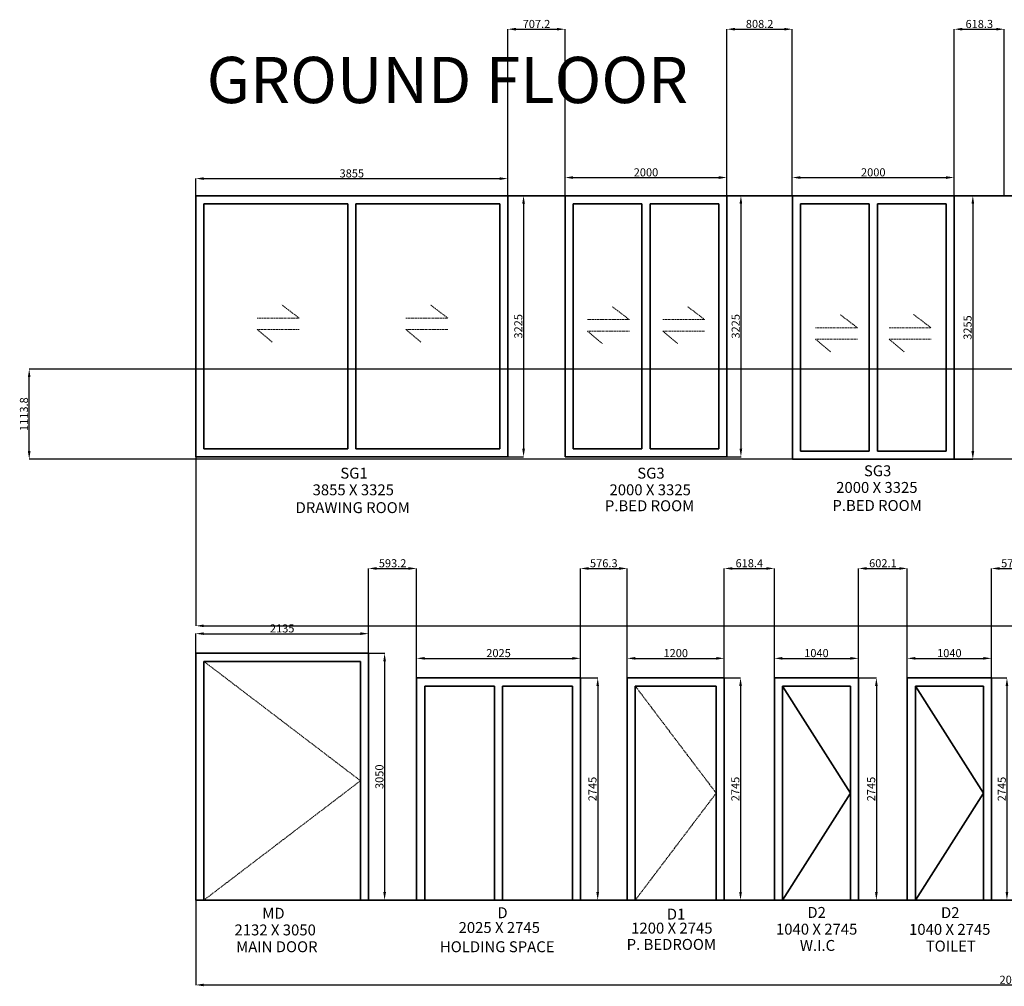
# Model space of a CAD drawing. Units: millimetres. Extents: x -850 to 42148, y -7352 to 4589.
# Tile 1 of 4: x -850 to 11314, y -7352 to 4589. Entities that reach past the tile are written whole.
import ezdxf

# ---------------------------------------------------------------- set-up
doc = ezdxf.new("R2010")
doc.units = ezdxf.units.MM
doc.linetypes.add('DASHED', pattern=[19.05, 12.7, -6.35])
for name, color, linetype, lineweight in [('A-ANNO-DIMS', 2, 'Continuous', 18), ('A-ANNO-TEXT', 7, 'Continuous', 18), ('A-DOOR', 3, 'Continuous', 35), ('A-DOOR-OPNG', 3, 'DASHED', 18), ('A-GLAZ', 4, 'Continuous', 35), ('A-GLAZ-OPNG', 4, 'DASHED', 18)]:
    doc.layers.add(name, color=color, linetype=linetype, lineweight=lineweight)
doc.styles.get("Standard").update_dxf_attribs({"font": 'arial.ttf'})
doc.dimstyles.new('ISO-25', dxfattribs={"dimtxt": 100, "dimasz": 100, "dimexe": 1.25, "dimexo": 0.625, "dimtad": 1, "dimtxsty": 'Standard', "dimcen": 2.5, "dimadec": 0, "dimazin": 0, "dimtfac": 1, "dimtmove": 0, "dimatfit": 3, "dimfxl": 1, "dimarcsym": 0})

# ---------------------------------------------------------------- blocks, each defined once
blk = doc.blocks.new('*D1')
at = {"layer": 'A-ANNO-DIMS', "color": 0, "lineweight": -2, "transparency": 16777216}
for p, q in [((1325, 2415), (1325, 2627)), ((1425, 2626), (5080, 2626)), ((5180, 2415), (5180, 2627))]:
    blk.add_line(p, q, dxfattribs=at)
at = {"layer": 'A-ANNO-DIMS', "color": 0, "lineweight": 30, "transparency": 16777216}
for points in [[(1425, 2642), (1425, 2609), (1325, 2626)], [(5080, 2642), (5080, 2609), (5180, 2626)]]:
    blk.add_solid(points, dxfattribs=at)
at = {"layer": 'Defpoints', "color": 0, "lineweight": 30, "transparency": 16777216}
for p in [(5180, 2626), (1325, 2414), (5180, 2414)]:
    blk.add_point(p, dxfattribs=at)
at = {"layer": 'A-ANNO-DIMS', "color": 0, "transparency": 16777216, "insert": (3253, 2677), "char_height": 100, "attachment_point": 5}
blk.add_mtext('3855', dxfattribs=at)
blk = doc.blocks.new('*D2')
at = {"layer": 'A-ANNO-DIMS', "color": 0, "lineweight": -2, "transparency": 16777216}
for p, q in [((5181, 2414), (5376, 2414)), ((5375, 2314), (5375, -711)), ((5181, -811), (5376, -811))]:
    blk.add_line(p, q, dxfattribs=at)
at = {"layer": 'A-ANNO-DIMS', "color": 0, "lineweight": 30, "transparency": 16777216}
for points in [[(5358, 2314), (5392, 2314), (5375, 2414)], [(5358, -711), (5392, -711), (5375, -811)]]:
    blk.add_solid(points, dxfattribs=at)
at = {"layer": 'Defpoints', "color": 0, "lineweight": 30, "transparency": 16777216}
for p in [(5180, 2414), (5180, -811), (5375, -811)]:
    blk.add_point(p, dxfattribs=at)
at = {"layer": 'A-ANNO-DIMS', "color": 0, "transparency": 16777216, "insert": (5323, 801), "char_height": 100, "attachment_point": 5, "rotation": 90}
blk.add_mtext('3225', dxfattribs=at)
blk = doc.blocks.new('*D3')
at = {"layer": 'A-ANNO-DIMS', "color": 0, "lineweight": -2, "transparency": 16777216}
for p, q in [((5887, 2415), (5887, 2640)), ((5987, 2639), (7787, 2639)), ((7887, 2415), (7887, 2640))]:
    blk.add_line(p, q, dxfattribs=at)
at = {"layer": 'A-ANNO-DIMS', "color": 0, "lineweight": 30, "transparency": 16777216}
for points in [[(5987, 2655), (5987, 2622), (5887, 2639)], [(7787, 2655), (7787, 2622), (7887, 2639)]]:
    blk.add_solid(points, dxfattribs=at)
at = {"layer": 'Defpoints', "color": 0, "lineweight": 30, "transparency": 16777216}
for p in [(7887, 2639), (5887, 2414), (7887, 2414)]:
    blk.add_point(p, dxfattribs=at)
at = {"layer": 'A-ANNO-DIMS', "color": 0, "transparency": 16777216, "insert": (6887, 2690), "char_height": 100, "attachment_point": 5}
blk.add_mtext('2000', dxfattribs=at)
blk = doc.blocks.new('*D4')
at = {"layer": 'A-ANNO-DIMS', "color": 0, "lineweight": -2, "transparency": 16777216}
for p, q in [((7888, 2414), (8061, 2414)), ((8060, 2314), (8060, -711)), ((7888, -811), (8061, -811))]:
    blk.add_line(p, q, dxfattribs=at)
at = {"layer": 'A-ANNO-DIMS', "color": 0, "lineweight": 30, "transparency": 16777216}
for points in [[(8043, 2314), (8076, 2314), (8060, 2414)], [(8043, -711), (8076, -711), (8060, -811)]]:
    blk.add_solid(points, dxfattribs=at)
at = {"layer": 'Defpoints', "color": 0, "lineweight": 30, "transparency": 16777216}
for p in [(7887, 2414), (7887, -811), (8060, -811)]:
    blk.add_point(p, dxfattribs=at)
at = {"layer": 'A-ANNO-DIMS', "color": 0, "transparency": 16777216, "insert": (8008, 801), "char_height": 100, "attachment_point": 5, "rotation": 90}
blk.add_mtext('3225', dxfattribs=at)
blk = doc.blocks.new('*D5')
at = {"layer": 'A-ANNO-DIMS', "color": 0, "lineweight": -2, "transparency": 16777216}
for p, q in [((8695, 2415), (8695, 2640)), ((8795, 2639), (10595, 2639)), ((10695, 2415), (10695, 2640))]:
    blk.add_line(p, q, dxfattribs=at)
at = {"layer": 'A-ANNO-DIMS', "color": 0, "lineweight": 30, "transparency": 16777216}
for points in [[(8795, 2655), (8795, 2622), (8695, 2639)], [(10595, 2655), (10595, 2622), (10695, 2639)]]:
    blk.add_solid(points, dxfattribs=at)
at = {"layer": 'Defpoints', "color": 0, "lineweight": 30, "transparency": 16777216}
for p in [(10695, 2639), (8695, 2414), (10695, 2414)]:
    blk.add_point(p, dxfattribs=at)
at = {"layer": 'A-ANNO-DIMS', "color": 0, "transparency": 16777216, "insert": (9695, 2690), "char_height": 100, "attachment_point": 5}
blk.add_mtext('2000', dxfattribs=at)
blk = doc.blocks.new('*D6')
at = {"layer": 'A-ANNO-DIMS', "color": 0, "lineweight": -2, "transparency": 16777216}
for p, q in [((10696, 2414), (10926, 2414)), ((10925, 2314), (10925, -741)), ((10696, -841), (10926, -841))]:
    blk.add_line(p, q, dxfattribs=at)
at = {"layer": 'A-ANNO-DIMS', "color": 0, "lineweight": 30, "transparency": 16777216}
for points in [[(10908, 2314), (10942, 2314), (10925, 2414)], [(10908, -741), (10942, -741), (10925, -841)]]:
    blk.add_solid(points, dxfattribs=at)
at = {"layer": 'Defpoints', "color": 0, "lineweight": 30, "transparency": 16777216}
for p in [(10695, 2414), (10695, -841), (10925, -841)]:
    blk.add_point(p, dxfattribs=at)
at = {"layer": 'A-ANNO-DIMS', "color": 0, "transparency": 16777216, "insert": (10873, 786), "char_height": 100, "attachment_point": 5, "rotation": 90}
blk.add_mtext('3255', dxfattribs=at)
blk = doc.blocks.new('*D29')
at = {"layer": 'A-ANNO-DIMS', "color": 0, "lineweight": -2, "transparency": 16777216}
for p, q in [((1325, -3237), (1325, -2994)), ((1425, -2996), (3360, -2996)), ((3460, -3237), (3460, -2994))]:
    blk.add_line(p, q, dxfattribs=at)
at = {"layer": 'A-ANNO-DIMS', "color": 0, "lineweight": 30, "transparency": 16777216}
for points in [[(1425, -2979), (1425, -3012), (1325, -2996)], [(3360, -2979), (3360, -3012), (3460, -2996)]]:
    blk.add_solid(points, dxfattribs=at)
at = {"layer": 'Defpoints', "color": 0, "lineweight": 30, "transparency": 16777216}
for p in [(3460, -2996), (1325, -3238), (3460, -3238)]:
    blk.add_point(p, dxfattribs=at)
at = {"layer": 'A-ANNO-DIMS', "color": 0, "transparency": 16777216, "insert": (2393, -2944), "char_height": 100, "attachment_point": 5}
blk.add_mtext('2135', dxfattribs=at)
blk = doc.blocks.new('*D30')
at = {"layer": 'A-ANNO-DIMS', "color": 0, "lineweight": -2, "transparency": 16777216}
for p, q in [((3461, -3238), (3660, -3238)), ((3658, -3338), (3658, -6188)), ((3461, -6288), (3660, -6288))]:
    blk.add_line(p, q, dxfattribs=at)
at = {"layer": 'A-ANNO-DIMS', "color": 0, "lineweight": 30, "transparency": 16777216}
for points in [[(3642, -3338), (3675, -3338), (3658, -3238)], [(3642, -6188), (3675, -6188), (3658, -6288)]]:
    blk.add_solid(points, dxfattribs=at)
at = {"layer": 'Defpoints', "color": 0, "lineweight": 30, "transparency": 16777216}
for p in [(3460, -3238), (3460, -6288), (3658, -6288)]:
    blk.add_point(p, dxfattribs=at)
at = {"layer": 'A-ANNO-DIMS', "color": 0, "transparency": 16777216, "insert": (3607, -4763), "char_height": 100, "attachment_point": 5, "rotation": 90}
blk.add_mtext('3050', dxfattribs=at)
blk = doc.blocks.new('*D31')
at = {"layer": 'A-ANNO-DIMS', "color": 0, "lineweight": -2, "transparency": 16777216}
for p, q in [((4053, -3542), (4053, -3299)), ((4153, -3301), (5978, -3301)), ((6078, -3542), (6078, -3299))]:
    blk.add_line(p, q, dxfattribs=at)
at = {"layer": 'A-ANNO-DIMS', "color": 0, "lineweight": 30, "transparency": 16777216}
for points in [[(4153, -3284), (4153, -3317), (4053, -3301)], [(5978, -3284), (5978, -3317), (6078, -3301)]]:
    blk.add_solid(points, dxfattribs=at)
at = {"layer": 'Defpoints', "color": 0, "lineweight": 30, "transparency": 16777216}
for p in [(6078, -3301), (4053, -3543), (6078, -3543)]:
    blk.add_point(p, dxfattribs=at)
at = {"layer": 'A-ANNO-DIMS', "color": 0, "transparency": 16777216, "insert": (5066, -3249), "char_height": 100, "attachment_point": 5}
blk.add_mtext('2025', dxfattribs=at)
blk = doc.blocks.new('*D32')
at = {"layer": 'A-ANNO-DIMS', "color": 0, "lineweight": -2, "transparency": 16777216}
for p, q in [((6079, -3543), (6292, -3543)), ((6291, -3643), (6291, -6188)), ((6079, -6288), (6292, -6288))]:
    blk.add_line(p, q, dxfattribs=at)
at = {"layer": 'A-ANNO-DIMS', "color": 0, "lineweight": 30, "transparency": 16777216}
for points in [[(6274, -3643), (6307, -3643), (6291, -3543)], [(6274, -6188), (6307, -6188), (6291, -6288)]]:
    blk.add_solid(points, dxfattribs=at)
at = {"layer": 'Defpoints', "color": 0, "lineweight": 30, "transparency": 16777216}
for p in [(6078, -3543), (6078, -6288), (6291, -6288)]:
    blk.add_point(p, dxfattribs=at)
at = {"layer": 'A-ANNO-DIMS', "color": 0, "transparency": 16777216, "insert": (6239, -4915), "char_height": 100, "attachment_point": 5, "rotation": 90}
blk.add_mtext('2745', dxfattribs=at)
blk = doc.blocks.new('*D33')
at = {"layer": 'A-ANNO-DIMS', "color": 0, "lineweight": -2, "transparency": 16777216}
for p, q in [((6655, -3542), (6655, -3299)), ((6755, -3301), (7755, -3301)), ((7855, -3542), (7855, -3299))]:
    blk.add_line(p, q, dxfattribs=at)
at = {"layer": 'A-ANNO-DIMS', "color": 0, "lineweight": 30, "transparency": 16777216}
for points in [[(6755, -3284), (6755, -3317), (6655, -3301)], [(7755, -3284), (7755, -3317), (7855, -3301)]]:
    blk.add_solid(points, dxfattribs=at)
at = {"layer": 'Defpoints', "color": 0, "lineweight": 30, "transparency": 16777216}
for p in [(7855, -3301), (6655, -3543), (7855, -3543)]:
    blk.add_point(p, dxfattribs=at)
at = {"layer": 'A-ANNO-DIMS', "color": 0, "transparency": 16777216, "insert": (7255, -3249), "char_height": 100, "attachment_point": 5}
blk.add_mtext('1200', dxfattribs=at)
blk = doc.blocks.new('*D34')
at = {"layer": 'A-ANNO-DIMS', "color": 0, "lineweight": -2, "transparency": 16777216}
for p, q in [((7855, -3543), (8056, -3543)), ((8055, -3643), (8055, -6188)), ((7855, -6288), (8056, -6288))]:
    blk.add_line(p, q, dxfattribs=at)
at = {"layer": 'A-ANNO-DIMS', "color": 0, "lineweight": 30, "transparency": 16777216}
for points in [[(8039, -3643), (8072, -3643), (8055, -3543)], [(8039, -6188), (8072, -6188), (8055, -6288)]]:
    blk.add_solid(points, dxfattribs=at)
at = {"layer": 'Defpoints', "color": 0, "lineweight": 30, "transparency": 16777216}
for p in [(7855, -3543), (7855, -6288), (8055, -6288)]:
    blk.add_point(p, dxfattribs=at)
at = {"layer": 'A-ANNO-DIMS', "color": 0, "transparency": 16777216, "insert": (8004, -4915), "char_height": 100, "attachment_point": 5, "rotation": 90}
blk.add_mtext('2745', dxfattribs=at)
blk = doc.blocks.new('*D35')
at = {"layer": 'A-ANNO-DIMS', "color": 0, "lineweight": -2, "transparency": 16777216}
for p, q in [((8473, -3542), (8473, -3299)), ((8573, -3301), (9413, -3301)), ((9513, -3542), (9513, -3299))]:
    blk.add_line(p, q, dxfattribs=at)
at = {"layer": 'A-ANNO-DIMS', "color": 0, "lineweight": 30, "transparency": 16777216}
for points in [[(8573, -3284), (8573, -3317), (8473, -3301)], [(9413, -3284), (9413, -3317), (9513, -3301)]]:
    blk.add_solid(points, dxfattribs=at)
at = {"layer": 'Defpoints', "color": 0, "lineweight": 30, "transparency": 16777216}
for p in [(9513, -3301), (8473, -3543), (9513, -3543)]:
    blk.add_point(p, dxfattribs=at)
at = {"layer": 'A-ANNO-DIMS', "color": 0, "transparency": 16777216, "insert": (8993, -3249), "char_height": 100, "attachment_point": 5}
blk.add_mtext('1040', dxfattribs=at)
blk = doc.blocks.new('*D36')
at = {"layer": 'A-ANNO-DIMS', "color": 0, "lineweight": -2, "transparency": 16777216}
for p, q in [((9514, -3543), (9735, -3543)), ((9733, -3643), (9733, -6188)), ((9514, -6288), (9735, -6288))]:
    blk.add_line(p, q, dxfattribs=at)
at = {"layer": 'A-ANNO-DIMS', "color": 0, "lineweight": 30, "transparency": 16777216}
for points in [[(9717, -3643), (9750, -3643), (9733, -3543)], [(9717, -6188), (9750, -6188), (9733, -6288)]]:
    blk.add_solid(points, dxfattribs=at)
at = {"layer": 'Defpoints', "color": 0, "lineweight": 30, "transparency": 16777216}
for p in [(9513, -3543), (9513, -6288), (9733, -6288)]:
    blk.add_point(p, dxfattribs=at)
at = {"layer": 'A-ANNO-DIMS', "color": 0, "transparency": 16777216, "insert": (9682, -4915), "char_height": 100, "attachment_point": 5, "rotation": 90}
blk.add_mtext('2745', dxfattribs=at)
blk = doc.blocks.new('*D37')
at = {"layer": 'A-ANNO-DIMS', "color": 0, "lineweight": -2, "transparency": 16777216}
for p, q in [((10115, -3542), (10115, -3299)), ((10215, -3301), (11055, -3301)), ((11155, -3542), (11155, -3299))]:
    blk.add_line(p, q, dxfattribs=at)
at = {"layer": 'A-ANNO-DIMS', "color": 0, "lineweight": 30, "transparency": 16777216}
for points in [[(10215, -3284), (10215, -3317), (10115, -3301)], [(11055, -3284), (11055, -3317), (11155, -3301)]]:
    blk.add_solid(points, dxfattribs=at)
at = {"layer": 'Defpoints', "color": 0, "lineweight": 30, "transparency": 16777216}
for p in [(11155, -3301), (10115, -3543), (11155, -3543)]:
    blk.add_point(p, dxfattribs=at)
at = {"layer": 'A-ANNO-DIMS', "color": 0, "transparency": 16777216, "insert": (10635, -3249), "char_height": 100, "attachment_point": 5}
blk.add_mtext('1040', dxfattribs=at)
blk = doc.blocks.new('*D38')
at = {"layer": 'A-ANNO-DIMS', "color": 0, "lineweight": -2, "transparency": 16777216}
for p, q in [((11156, -3543), (11347, -3543)), ((11346, -3643), (11346, -6188)), ((11156, -6288), (11347, -6288))]:
    blk.add_line(p, q, dxfattribs=at)
at = {"layer": 'A-ANNO-DIMS', "color": 0, "lineweight": 30, "transparency": 16777216}
for points in [[(11330, -3643), (11363, -3643), (11346, -3543)], [(11330, -6188), (11363, -6188), (11346, -6288)]]:
    blk.add_solid(points, dxfattribs=at)
at = {"layer": 'Defpoints', "color": 0, "lineweight": 30, "transparency": 16777216}
for p in [(11155, -3543), (11155, -6288), (11346, -6288)]:
    blk.add_point(p, dxfattribs=at)
at = {"layer": 'A-ANNO-DIMS', "color": 0, "transparency": 16777216, "insert": (11295, -4915), "char_height": 100, "attachment_point": 5, "rotation": 90}
blk.add_mtext('2745', dxfattribs=at)
blk = doc.blocks.new('SYM-SLIDE-ARROW')
for p, q in [((2602, 903), (2388, 1066)), ((2084, 903), (2602, 903)), ((2085, 760), (2604, 760)), ((2085, 760), (2269, 607))]:
    blk.add_line(p, q)
blk = doc.blocks.new('DOOR-D2-1040')
for p, q in [((8473, -6288), (8473, -3543)), ((8473, -3543), (9513, -3543)), ((8573, -6288), (8573, -3643)), ((8573, -3643), (9413, -3643)), ((8573, -3643), (9413, -4965)), ((9413, -3643), (9413, -6288)), ((9513, -3543), (9513, -6288)), ((9413, -4965), (8573, -6288))]:
    blk.add_line(p, q)
blk = doc.blocks.new('*D60')
at = {"layer": 'A-ANNO-DIMS', "color": 0, "lineweight": -2, "transparency": 16777216}
for p, q in [((41489, -432), (41489, -2900)), ((1325, -812), (1325, -2900)), ((1425, -2899), (41389, -2899))]:
    blk.add_line(p, q, dxfattribs=at)
at = {"layer": 'A-ANNO-DIMS', "color": 0, "lineweight": 30, "transparency": 16777216}
for points in [[(1425, -2882), (1425, -2915), (1325, -2899)], [(41389, -2882), (41389, -2915), (41489, -2899)]]:
    blk.add_solid(points, dxfattribs=at)
at = {"layer": 'Defpoints', "color": 0, "lineweight": 30, "transparency": 16777216}
for p in [(41489, -431), (1325, -811), (41489, -2899)]:
    blk.add_point(p, dxfattribs=at)
at = {"layer": 'A-ANNO-DIMS', "color": 0, "transparency": 16777216, "insert": (21407, -2847), "char_height": 100, "attachment_point": 5}
blk.add_mtext('40164', dxfattribs=at)
blk = doc.blocks.new('*D61')
at = {"layer": 'A-ANNO-DIMS', "color": 0, "lineweight": -2, "transparency": 16777216}
for p, q in [((5180, 2415), (5180, 4473)), ((5280, 4471), (5787, 4471)), ((5887, 2415), (5887, 4473))]:
    blk.add_line(p, q, dxfattribs=at)
at = {"layer": 'A-ANNO-DIMS', "color": 0, "lineweight": 30, "transparency": 16777216}
for points in [[(5280, 4488), (5280, 4455), (5180, 4471)], [(5787, 4488), (5787, 4455), (5887, 4471)]]:
    blk.add_solid(points, dxfattribs=at)
at = {"layer": 'Defpoints', "color": 0, "lineweight": 30, "transparency": 16777216}
for p in [(5887, 4471), (5180, 2414), (5887, 2414)]:
    blk.add_point(p, dxfattribs=at)
at = {"layer": 'A-ANNO-DIMS', "color": 0, "transparency": 16777216, "insert": (5534, 4523), "char_height": 100, "attachment_point": 5}
blk.add_mtext('707.2', dxfattribs=at)
blk = doc.blocks.new('*D62')
at = {"layer": 'A-ANNO-DIMS', "color": 0, "lineweight": -2, "transparency": 16777216}
for p, q in [((7887, 2415), (7887, 4473)), ((7987, 4471), (8595, 4471)), ((8695, 2415), (8695, 4473))]:
    blk.add_line(p, q, dxfattribs=at)
at = {"layer": 'A-ANNO-DIMS', "color": 0, "lineweight": 30, "transparency": 16777216}
for points in [[(7987, 4488), (7987, 4455), (7887, 4471)], [(8595, 4488), (8595, 4455), (8695, 4471)]]:
    blk.add_solid(points, dxfattribs=at)
at = {"layer": 'Defpoints', "color": 0, "lineweight": 30, "transparency": 16777216}
for p in [(8695, 4471), (7887, 2414), (8695, 2414)]:
    blk.add_point(p, dxfattribs=at)
at = {"layer": 'A-ANNO-DIMS', "color": 0, "transparency": 16777216, "insert": (8291, 4523), "char_height": 100, "attachment_point": 5}
blk.add_mtext('808.2', dxfattribs=at)
blk = doc.blocks.new('*D63')
at = {"layer": 'A-ANNO-DIMS', "color": 0, "lineweight": -2, "transparency": 16777216}
for p, q in [((10695, 2415), (10695, 4473)), ((10795, 4471), (11214, 4471)), ((11314, 2415), (11314, 4473))]:
    blk.add_line(p, q, dxfattribs=at)
at = {"layer": 'A-ANNO-DIMS', "color": 0, "lineweight": 30, "transparency": 16777216}
for points in [[(10795, 4488), (10795, 4455), (10695, 4471)], [(11214, 4488), (11214, 4455), (11314, 4471)]]:
    blk.add_solid(points, dxfattribs=at)
at = {"layer": 'Defpoints', "color": 0, "lineweight": 30, "transparency": 16777216}
for p in [(11314, 4471), (10695, 2414), (11314, 2414)]:
    blk.add_point(p, dxfattribs=at)
at = {"layer": 'A-ANNO-DIMS', "color": 0, "transparency": 16777216, "insert": (11005, 4523), "char_height": 100, "attachment_point": 5}
blk.add_mtext('618.3', dxfattribs=at)
blk = doc.blocks.new('*D74')
at = {"layer": 'A-ANNO-DIMS', "color": 0, "lineweight": -2, "transparency": 16777216}
for p, q in [((17345, 273), (-734, 273)), ((-732, -741), (-732, 173)), ((17245, -841), (-734, -841))]:
    blk.add_line(p, q, dxfattribs=at)
at = {"layer": 'A-ANNO-DIMS', "color": 0, "lineweight": 30, "transparency": 16777216}
for points in [[(-749, 173), (-716, 173), (-732, 273)], [(-749, -741), (-716, -741), (-732, -841)]]:
    blk.add_solid(points, dxfattribs=at)
at = {"layer": 'Defpoints', "color": 0, "lineweight": 30, "transparency": 16777216}
for p in [(-732, 273), (17346, 273), (17246, -841)]:
    blk.add_point(p, dxfattribs=at)
at = {"layer": 'A-ANNO-DIMS', "color": 0, "transparency": 16777216, "insert": (-784, -284), "char_height": 100, "attachment_point": 5, "rotation": 90}
blk.add_mtext('1113.8', dxfattribs=at)
blk = doc.blocks.new('*D83')
at = {"layer": 'A-ANNO-DIMS', "color": 0, "lineweight": -2, "transparency": 16777216}
for p, q in [((1325, -3238), (1325, -7337)), ((21562, -6288), (21562, -7337)), ((1425, -7335), (21462, -7335))]:
    blk.add_line(p, q, dxfattribs=at)
at = {"layer": 'A-ANNO-DIMS', "color": 0, "lineweight": 30, "transparency": 16777216}
for points in [[(1425, -7319), (1425, -7352), (1325, -7335)], [(21462, -7319), (21462, -7352), (21562, -7335)]]:
    blk.add_solid(points, dxfattribs=at)
at = {"layer": 'Defpoints', "color": 0, "lineweight": 30, "transparency": 16777216}
for p in [(1325, -3238), (21562, -6288), (21562, -7335)]:
    blk.add_point(p, dxfattribs=at)
at = {"layer": 'A-ANNO-DIMS', "color": 0, "transparency": 16777216, "insert": (11444, -7284), "char_height": 100, "attachment_point": 5}
blk.add_mtext('20237', dxfattribs=at)
blk = doc.blocks.new('*D84')
at = {"layer": 'A-ANNO-DIMS', "color": 0, "lineweight": -2, "transparency": 16777216}
for p, q in [((3460, -3237), (3460, -2189)), ((4053, -3542), (4053, -2189)), ((3560, -2190), (3953, -2190))]:
    blk.add_line(p, q, dxfattribs=at)
at = {"layer": 'A-ANNO-DIMS', "color": 0, "lineweight": 30, "transparency": 16777216}
for points in [[(3560, -2174), (3560, -2207), (3460, -2190)], [(3953, -2174), (3953, -2207), (4053, -2190)]]:
    blk.add_solid(points, dxfattribs=at)
at = {"layer": 'Defpoints', "color": 0, "lineweight": 30, "transparency": 16777216}
for p in [(4053, -2190), (3460, -3238), (4053, -3543)]:
    blk.add_point(p, dxfattribs=at)
at = {"layer": 'A-ANNO-DIMS', "color": 0, "transparency": 16777216, "insert": (3757, -2139), "char_height": 100, "attachment_point": 5}
blk.add_mtext('593.2', dxfattribs=at)
blk = doc.blocks.new('*D85')
at = {"layer": 'A-ANNO-DIMS', "color": 0, "lineweight": -2, "transparency": 16777216}
for p, q in [((6078, -3542), (6078, -2189)), ((6655, -3542), (6655, -2189)), ((6178, -2190), (6555, -2190))]:
    blk.add_line(p, q, dxfattribs=at)
at = {"layer": 'A-ANNO-DIMS', "color": 0, "lineweight": 30, "transparency": 16777216}
for points in [[(6178, -2174), (6178, -2207), (6078, -2190)], [(6555, -2174), (6555, -2207), (6655, -2190)]]:
    blk.add_solid(points, dxfattribs=at)
at = {"layer": 'Defpoints', "color": 0, "lineweight": 30, "transparency": 16777216}
for p in [(6655, -2190), (6078, -3543), (6655, -3543)]:
    blk.add_point(p, dxfattribs=at)
at = {"layer": 'A-ANNO-DIMS', "color": 0, "transparency": 16777216, "insert": (6366, -2139), "char_height": 100, "attachment_point": 5}
blk.add_mtext('576.3', dxfattribs=at)
blk = doc.blocks.new('*D86')
at = {"layer": 'A-ANNO-DIMS', "color": 0, "lineweight": -2, "transparency": 16777216}
for p, q in [((7855, -3542), (7855, -2189)), ((8473, -3542), (8473, -2189)), ((7955, -2190), (8373, -2190))]:
    blk.add_line(p, q, dxfattribs=at)
at = {"layer": 'A-ANNO-DIMS', "color": 0, "lineweight": 30, "transparency": 16777216}
for points in [[(7955, -2174), (7955, -2207), (7855, -2190)], [(8373, -2174), (8373, -2207), (8473, -2190)]]:
    blk.add_solid(points, dxfattribs=at)
at = {"layer": 'Defpoints', "color": 0, "lineweight": 30, "transparency": 16777216}
for p in [(8473, -2190), (7855, -3543), (8473, -3543)]:
    blk.add_point(p, dxfattribs=at)
at = {"layer": 'A-ANNO-DIMS', "color": 0, "transparency": 16777216, "insert": (8164, -2139), "char_height": 100, "attachment_point": 5}
blk.add_mtext('618.4', dxfattribs=at)
blk = doc.blocks.new('*D87')
at = {"layer": 'A-ANNO-DIMS', "color": 0, "lineweight": -2, "transparency": 16777216}
for p, q in [((9513, -3542), (9513, -2189)), ((10115, -3542), (10115, -2189)), ((9613, -2190), (10015, -2190))]:
    blk.add_line(p, q, dxfattribs=at)
at = {"layer": 'A-ANNO-DIMS', "color": 0, "lineweight": 30, "transparency": 16777216}
for points in [[(9613, -2174), (9613, -2207), (9513, -2190)], [(10015, -2174), (10015, -2207), (10115, -2190)]]:
    blk.add_solid(points, dxfattribs=at)
at = {"layer": 'Defpoints', "color": 0, "lineweight": 30, "transparency": 16777216}
for p in [(10115, -2190), (9513, -3543), (10115, -3543)]:
    blk.add_point(p, dxfattribs=at)
at = {"layer": 'A-ANNO-DIMS', "color": 0, "transparency": 16777216, "insert": (9814, -2139), "char_height": 100, "attachment_point": 5}
blk.add_mtext('602.1', dxfattribs=at)
blk = doc.blocks.new('*D88')
at = {"layer": 'A-ANNO-DIMS', "color": 0, "lineweight": -2, "transparency": 16777216}
for p, q in [((11155, -3542), (11155, -2189)), ((11734, -3542), (11734, -2189)), ((11255, -2190), (11634, -2190))]:
    blk.add_line(p, q, dxfattribs=at)
at = {"layer": 'A-ANNO-DIMS', "color": 0, "lineweight": 30, "transparency": 16777216}
for points in [[(11255, -2174), (11255, -2207), (11155, -2190)], [(11634, -2174), (11634, -2207), (11734, -2190)]]:
    blk.add_solid(points, dxfattribs=at)
at = {"layer": 'Defpoints', "color": 0, "lineweight": 30, "transparency": 16777216}
for p in [(11734, -2190), (11155, -3543), (11734, -3543)]:
    blk.add_point(p, dxfattribs=at)
at = {"layer": 'A-ANNO-DIMS', "color": 0, "transparency": 16777216, "insert": (11445, -2139), "char_height": 100, "attachment_point": 5}
blk.add_mtext('579.2', dxfattribs=at)

msp = doc.modelspace()

# ---------------------------------------------------------------- linework, layer by layer
at = {"layer": 'A-DOOR'}
for p, q in [((1325.061, -3237.868), (1325.061, -6287.868)), ((3460.061, -3237.868), (1325.061, -3237.868)), ((3460.061, -6287.868), (3460.061, -3237.868)), ((1425.061, -3337.868), (1425.061, -6287.868)), ((1425.061, -3337.868), (3360.061, -3337.868)), ((3360.061, -6287.868), (3360.061, -3337.868)), ((4053.252, -3542.868), (4053.252, -6287.868)), ((6078.252, -3542.868), (4053.252, -3542.868)), ((4153.252, -3642.868), (4153.252, -6287.868)), ((4153.252, -3642.868), (5015.752, -3642.868)), ((5015.752, -6287.868), (5015.752, -3642.868)), ((5115.752, -6287.868), (5115.752, -3642.868)), ((5115.752, -3642.868), (5978.252, -3642.868)), ((5978.252, -6287.868), (5978.252, -3642.868)), ((6078.252, -6287.868), (6078.252, -3542.868)), ((6654.512, -3542.868), (6654.512, -6287.868)), ((6654.512, -3542.868), (7854.512, -3542.868)), ((6754.512, -3642.868), (7754.512, -3642.868)), ((6754.512, -3642.868), (6754.512, -6287.868)), ((7754.512, -6287.868), (7754.512, -3642.868)), ((7854.512, -6287.868), (7854.512, -3542.868)), ((1325.061, -6287.868), (3460.061, -6287.868)), ((1325.061, -6287.868), (21721.958, -6287.868)), ((1425.061, -6287.868), (3360.061, -6287.868)), ((4053.252, -6287.868), (6078.252, -6287.868)), ((4153.252, -6287.868), (5015.752, -6287.868)), ((5115.752, -6287.868), (5978.252, -6287.868)), ((6654.512, -6287.868), (7854.512, -6287.868))]:
    msp.add_line(p, q, dxfattribs=at)
at = {"layer": 'A-DOOR-OPNG'}
for p, q in [((1425.061, -3337.868), (3360.061, -4812.868)), ((6754.512, -3642.868), (7754.512, -4965.368)), ((3360.061, -4812.868), (1425.061, -6287.868)), ((7754.512, -4965.368), (6754.512, -6287.868))]:
    msp.add_line(p, q, dxfattribs=at)
at = {"layer": 'A-GLAZ'}
for p, q in [((1325.061, 2413.876), (15141.402, 2413.876)), ((1325.061, 2413.876), (1325.061, -811.124)), ((1425.061, 2313.876), (1425.061, -711.124)), ((1425.061, 2313.876), (3202.561, 2313.876)), ((3202.561, -711.124), (3202.561, 2313.876)), ((3302.561, -711.124), (3302.561, 2313.876)), ((3302.561, 2313.876), (5080.061, 2313.876)), ((5080.061, -711.124), (5080.061, 2313.876)), ((5180.061, -811.124), (5180.061, 2413.876)), ((5887.297, 2413.876), (5887.297, -811.124)), ((5987.297, 2313.876), (5987.297, -711.124)), ((5987.297, 2313.876), (6837.297, 2313.876)), ((6837.297, -711.124), (6837.297, 2313.876)), ((6937.297, -711.124), (6937.297, 2313.876)), ((6937.297, 2313.876), (7787.297, 2313.876)), ((7787.297, -711.124), (7787.297, 2313.876)), ((7887.297, -811.124), (7887.297, 2413.876)), ((8695.469, 2413.876), (8695.469, -841.124)), ((8795.469, 2313.876), (8795.469, -741.124)), ((8795.469, 2313.876), (9645.469, 2313.876)), ((9645.469, -741.124), (9645.469, 2313.876)), ((9745.469, -741.124), (9745.469, 2313.876)), ((9745.469, 2313.876), (10595.469, 2313.876)), ((10595.469, -741.124), (10595.469, 2313.876)), ((10695.469, -841.124), (10695.469, 2413.876)), ((1425.061, -711.124), (3202.561, -711.124)), ((3302.561, -711.124), (5080.061, -711.124)), ((5987.297, -711.124), (6837.297, -711.124)), ((6937.297, -711.124), (7787.297, -711.124)), ((1325.061, -811.124), (5180.061, -811.124)), ((5887.297, -811.124), (7887.297, -811.124)), ((8695.469, -841.124), (10695.469, -841.124)), ((8795.469, -741.124), (9645.469, -741.124)), ((9745.469, -741.124), (10595.469, -741.124))]:
    msp.add_line(p, q, dxfattribs=at)

# ---------------------------------------------------------------- block references
at = {"layer": 'A-DOOR'}
for p in [(0, 0), (1642.144, 0)]:
    msp.add_blockref('DOOR-D2-1040', p, dxfattribs=at)
at = {"layer": 'A-GLAZ-OPNG'}
for p in [(0, 0), (1836.299, 0), (4079.84, -19.672), (5010.877, -19.672), (6896.819, -119.626), (7805.853, -119.626)]:
    msp.add_blockref('SYM-SLIDE-ARROW', p, dxfattribs=at)

# ---------------------------------------------------------------- texts
at = {"layer": 'A-ANNO-TEXT'}
for s, height, p in [('GROUND FLOOR ', 570.99867, (1459.848, 3558.528)), ('SG1', 134.8889, (3111.408, -1080.272)), ('SG3', 134.8889, (6779.382, -1080.272)), ('SG3', 134.8889, (9579.584, -1051.132)), ('3855 X 3325', 134.88886, (2768.634, -1286.109)), ('2000 X 3325', 134.88886, (6436.608, -1286.109)), ('2000 X 3325', 134.88886, (9236.811, -1256.969)), ('DRAWING ROOM', 134.88886, (2558.69, -1506.333)), ('P.BED ROOM', 134.8889, (6379.615, -1483.329)), ('P.BED ROOM', 134.8889, (9190.074, -1479.804)), ('MD', 134.8889, (2146.755, -6517.389)), ('D', 134.889, (5051.144, -6510.891)), ('D1', 134.8889, (7144.448, -6527.558)), ('D2', 134.8889, (8880.67, -6507.134)), ('D2', 134.8889, (10531.531, -6509.666)), ('2025 X 2745', 134.88886, (4572.184, -6693.317)), ('1200 X 2745', 134.88886, (6704.199, -6700.775)), ('2132 X 3050', 134.88886, (1803.981, -6723.226)), ('1040 X 2745', 134.88886, (8493.165, -6713.572)), ('1040 X 2745', 134.88886, (10137.24, -6716.19)), ('MAIN DOOR', 134.8889, (1823.91, -6930.692)), ('HOLDING SPACE', 134.88886, (4341.165, -6930.759)), ('P. BEDROOM', 134.8889, (6648.213, -6902.053)), ('W.I.C', 134.8889, (8788.285, -6914.764)), ('TOILET', 134.8889, (10343.405, -6922.488))]:
    msp.add_text(s, height=height, dxfattribs=at).set_placement(p)

# ---------------------------------------------------------------- dimensions: what is measured, and where the dimension line sits
at = {"layer": 'A-ANNO-DIMS'}
for base, p1, p2, override, picture, middle in [((5887.297, 4471.376), (5180.061, 2413.876), (5887.297, 2413.876), {"dimdec": 1, "dimlfac": 1, "dimrnd": 0, "dimzin": 0, "dimdsep": 46, "dimlunit": 2}, '*D61', (5533.679, 4523.058)), ((8695.469, 4471.376), (7887.297, 2413.876), (8695.469, 2413.876), {"dimdec": 1, "dimlfac": 1, "dimrnd": 0, "dimzin": 0, "dimdsep": 46, "dimlunit": 2}, '*D62', (8291.383, 4523.058)), ((11313.76, 4471.376), (10695.469, 2413.876), (11313.76, 2413.876), {"dimdec": 1, "dimlfac": 1, "dimrnd": 0, "dimzin": 0, "dimdsep": 46, "dimlunit": 2}, '*D63', (11004.614, 4523.092)), ((5180.061, 2625.75), (1325.061, 2413.876), (5180.061, 2413.876), {"dimclrd": 0, "dimclre": 0, "dimclrt": 0}, '*D1', (3252.561, 2677.466)), ((7887.297, 2638.596), (5887.297, 2413.876), (7887.297, 2413.876), {"dimclrd": 0, "dimclre": 0, "dimclrt": 0}, '*D3', (6887.297, 2690.278)), ((10695.469, 2638.596), (8695.469, 2413.876), (10695.469, 2413.876), {"dimclrd": 0, "dimclre": 0, "dimclrt": 0}, '*D5', (9695.469, 2690.278)), ((41488.766, -2898.624), (1325.061, -811.124), (41488.766, -431.124), {"dimdec": 0, "dimlfac": 1, "dimrnd": 0, "dimzin": 0, "dimdsep": 46, "dimlunit": 2}, '*D60', (21406.913, -2846.942)), ((4053.252, -2190.368), (3460.061, -3237.868), (4053.252, -3542.868), {"dimdec": 1, "dimlfac": 1, "dimrnd": 0, "dimzin": 0, "dimdsep": 46, "dimlunit": 2}, '*D84', (3756.656, -2138.651)), ((6654.512, -2190.368), (6078.252, -3542.868), (6654.512, -3542.868), {"dimdec": 1, "dimlfac": 1, "dimrnd": 0, "dimzin": 0, "dimdsep": 46, "dimlunit": 2}, '*D85', (6366.382, -2138.651)), ((8472.883, -2190.368), (7854.512, -3542.868), (8472.883, -3542.868), {"dimdec": 1, "dimlfac": 1, "dimrnd": 0, "dimzin": 0, "dimdsep": 46, "dimlunit": 2}, '*D86', (8163.697, -2138.685)), ((10115.027, -2190.368), (9512.883, -3542.868), (10115.027, -3542.868), {"dimdec": 1, "dimlfac": 1, "dimrnd": 0, "dimzin": 0, "dimdsep": 46, "dimlunit": 2}, '*D87', (9813.955, -2138.685)), ((11734.228, -2190.368), (11155.027, -3542.868), (11734.228, -3542.868), {"dimdec": 1, "dimlfac": 1, "dimrnd": 0, "dimzin": 0, "dimdsep": 46, "dimlunit": 2}, '*D88', (11444.627, -2138.685)), ((3460.061, -2995.609), (1325.061, -3237.868), (3460.061, -3237.868), {"dimclrd": 0, "dimclre": 0, "dimclrt": 0}, '*D29', (2392.561, -2943.892)), ((21561.986, -7335.368), (1325.061, -3237.868), (21561.986, -6287.868), {"dimdec": 0, "dimlfac": 1, "dimrnd": 0, "dimzin": 0, "dimdsep": 46, "dimlunit": 2}, '*D83', (11443.523, -7283.651)), ((6078.252, -3300.609), (4053.252, -3542.868), (6078.252, -3542.868), {"dimclrd": 0, "dimclre": 0, "dimclrt": 0}, '*D31', (5065.752, -3248.927)), ((7854.512, -3300.609), (6654.512, -3542.868), (7854.512, -3542.868), {"dimclrd": 0, "dimclre": 0, "dimclrt": 0}, '*D33', (7254.512, -3248.927)), ((9512.883, -3300.609), (8472.883, -3542.868), (9512.883, -3542.868), {"dimclrd": 0, "dimclre": 0, "dimclrt": 0}, '*D35', (8992.883, -3248.927)), ((11155.027, -3300.609), (10115.027, -3542.868), (11155.027, -3542.868), {"dimclrd": 0, "dimclre": 0, "dimclrt": 0}, '*D37', (10635.027, -3248.927))]:
    dim = msp.add_linear_dim(base=base, p1=p1, p2=p2, dimstyle='ISO-25', override=override, dxfattribs=at)
    dim.commit()
    dim.dimension.update_dxf_attribs({"geometry": picture, "text_midpoint": middle})
for base, p1, p2, override, picture, middle in [((5374.86, -811.124), (5180.061, 2413.876), (5180.061, -811.124), {"dimclrd": 0, "dimclre": 0, "dimclrt": 0}, '*D2', (5323.144, 801.376)), ((8059.83, -811.124), (7887.297, 2413.876), (7887.297, -811.124), {"dimclrd": 0, "dimclre": 0, "dimclrt": 0}, '*D4', (8008.114, 801.376)), ((10925.011, -841.124), (10695.469, 2413.876), (10695.469, -841.124), {"dimclrd": 0, "dimclre": 0, "dimclrt": 0}, '*D6', (10873.294, 786.376)), ((-732.439, 272.698), (17245.641, -841.124), (17345.641, 272.698), {"dimdec": 1, "dimlfac": 1, "dimrnd": 0, "dimzin": 0, "dimdsep": 46, "dimlunit": 2}, '*D74', (-784.156, -284.213)), ((3658.286, -6287.868), (3460.061, -3237.868), (3460.061, -6287.868), {"dimclrd": 0, "dimclre": 0, "dimclrt": 0}, '*D30', (3606.57, -4762.868)), ((6290.826, -6287.868), (6078.252, -3542.868), (6078.252, -6287.868), {"dimclrd": 0, "dimclre": 0, "dimclrt": 0}, '*D32', (6239.144, -4915.368)), ((8055.223, -6287.868), (7854.512, -3542.868), (7854.512, -6287.868), {"dimclrd": 0, "dimclre": 0, "dimclrt": 0}, '*D34', (8003.541, -4915.368)), ((9733.258, -6287.868), (9512.883, -3542.868), (9512.883, -6287.868), {"dimclrd": 0, "dimclre": 0, "dimclrt": 0}, '*D36', (9681.576, -4915.368)), ((11346.2, -6287.868), (11155.027, -3542.868), (11155.027, -6287.868), {"dimclrd": 0, "dimclre": 0, "dimclrt": 0}, '*D38', (11294.518, -4915.368))]:
    dim = msp.add_linear_dim(base=base, p1=p1, p2=p2, angle=90, dimstyle='ISO-25', override=override, dxfattribs=at)
    dim.commit()
    dim.dimension.update_dxf_attribs({"geometry": picture, "text_midpoint": middle})

doc.saveas('drawing.dxf')
